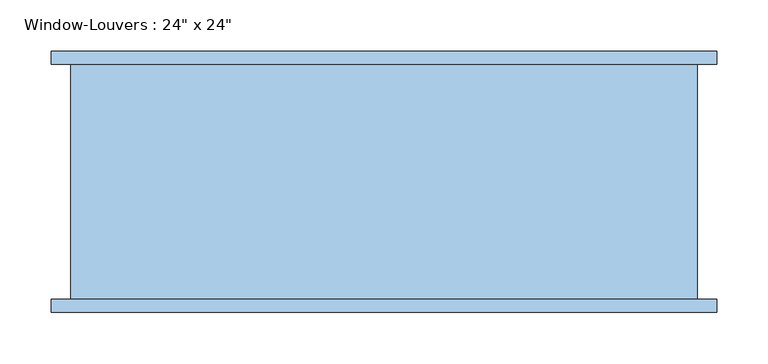
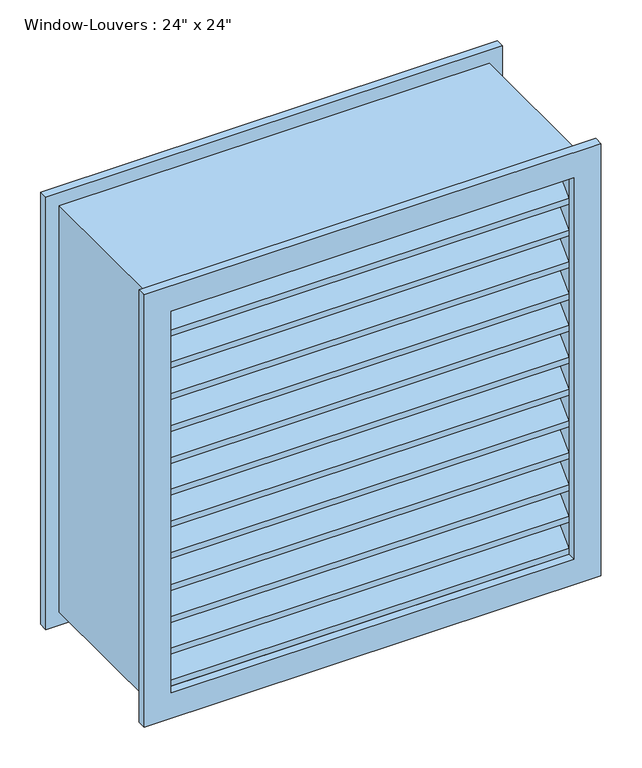
"""IFC4 building model written with IfcOpenShell, lengths in millimetres: window geometry."""

from ifc_helpers import new_model, si_unit, frame, origin, place, context, project, spatial, polyline, outline, extrude, source, transform, mapped, element, save


def window_407d3824(model_context):
    return source(origin(), model_context, "Body", "SweptSolid", [
        extrude(outline(polyline([(-107.95, 1419.1754778), (-69.85, 1457.2754778), (-31.75, 1419.1754778), (-31.75, 1410.1952217), (-69.85, 1448.2952217), (-107.95, 1410.1952217), (-107.95, 1419.1754778)])), frame((-285.75, 0.0, 0.0), z_axis=(1.0, 0.0, 0.0), x_axis=(0.0, 1.0, 0.0)), (0.0, 0.0, 1.0), 571.5),
        extrude(outline(polyline([(-107.95, 1371.5009557), (-69.85, 1409.6009557), (-31.75, 1371.5009557), (-31.75, 1362.5206995), (-69.85, 1400.6206995), (-107.95, 1362.5206995), (-107.95, 1371.5009557)])), frame((-285.75, 0.0, 0.0), z_axis=(1.0, 0.0, 0.0), x_axis=(0.0, 1.0, 0.0)), (0.0, 0.0, 1.0), 571.5),
        extrude(outline(polyline([(-107.95, 1323.8264335), (-69.85, 1361.9264335), (-31.75, 1323.8264335), (-31.75, 1314.8461774), (-69.85, 1352.9461774), (-107.95, 1314.8461774), (-107.95, 1323.8264335)])), frame((-285.75, 0.0, 0.0), z_axis=(1.0, 0.0, 0.0), x_axis=(0.0, 1.0, 0.0)), (0.0, 0.0, 1.0), 571.5),
        extrude(outline(polyline([(-107.95, 1276.1519113), (-69.85, 1314.2519113), (-31.75, 1276.1519113), (-31.75, 1267.1716552), (-69.85, 1305.2716552), (-107.95, 1267.1716552), (-107.95, 1276.1519113)])), frame((-285.75, 0.0, 0.0), z_axis=(1.0, 0.0, 0.0), x_axis=(0.0, 1.0, 0.0)), (0.0, 0.0, 1.0), 571.5),
        extrude(outline(polyline([(-107.95, 1228.4773891), (-69.85, 1266.5773891), (-31.75, 1228.4773891), (-31.75, 1219.497133), (-69.85, 1257.597133), (-107.95, 1219.497133), (-107.95, 1228.4773891)])), frame((-285.75, 0.0, 0.0), z_axis=(1.0, 0.0, 0.0), x_axis=(0.0, 1.0, 0.0)), (0.0, 0.0, 1.0), 571.5),
        extrude(outline(polyline([(-107.95, 1180.802867), (-69.85, 1218.902867), (-31.75, 1180.802867), (-31.75, 1171.8226109), (-69.85, 1209.9226109), (-107.95, 1171.8226109), (-107.95, 1180.802867)])), frame((-285.75, 0.0, 0.0), z_axis=(1.0, 0.0, 0.0), x_axis=(0.0, 1.0, 0.0)), (0.0, 0.0, 1.0), 571.5),
        extrude(outline(polyline([(-107.95, 1133.1283448), (-69.85, 1171.2283448), (-31.75, 1133.1283448), (-31.75, 1124.1480887), (-69.85, 1162.2480887), (-107.95, 1124.1480887), (-107.95, 1133.1283448)])), frame((-285.75, 0.0, 0.0), z_axis=(1.0, 0.0, 0.0), x_axis=(0.0, 1.0, 0.0)), (0.0, 0.0, 1.0), 571.5),
        extrude(outline(polyline([(-107.95, 1085.4538226), (-69.85, 1123.5538226), (-31.75, 1085.4538226), (-31.75, 1076.4735665), (-69.85, 1114.5735665), (-107.95, 1076.4735665), (-107.95, 1085.4538226)])), frame((-285.75, 0.0, 0.0), z_axis=(1.0, 0.0, 0.0), x_axis=(0.0, 1.0, 0.0)), (0.0, 0.0, 1.0), 571.5),
        extrude(outline(polyline([(-107.95, 1037.7793005), (-69.85, 1075.8793005), (-31.75, 1037.7793005), (-31.75, 1028.7990443), (-69.85, 1066.8990443), (-107.95, 1028.7990443), (-107.95, 1037.7793005)])), frame((-285.75, 0.0, 0.0), z_axis=(1.0, 0.0, 0.0), x_axis=(0.0, 1.0, 0.0)), (0.0, 0.0, 1.0), 571.5),
        extrude(outline(polyline([(-107.95, 990.1047783), (-69.85, 1028.2047783), (-31.75, 990.1047783), (-31.75, 981.1245222), (-69.85, 1019.2245222), (-107.95, 981.1245222), (-107.95, 990.1047783)])), frame((-285.75, 0.0, 0.0), z_axis=(1.0, 0.0, 0.0), x_axis=(0.0, 1.0, 0.0)), (0.0, 0.0, 1.0), 571.5),
        extrude(outline(polyline([(-107.95, 1466.85), (-69.85, 1504.95), (-31.75, 1466.85), (-31.75, 1457.8697439), (-69.85, 1495.9697439), (-107.95, 1457.8697439), (-107.95, 1466.85)])), frame((-285.75, 0.0, 0.0), z_axis=(1.0, 0.0, 0.0), x_axis=(0.0, 1.0, 0.0)), (0.0, 0.0, 1.0), 571.5),
        extrude(outline(polyline([(-107.95, 942.4302561), (-69.85, 980.5302561), (-31.75, 942.4302561), (-31.75, 933.45), (-69.85, 971.55), (-107.95, 933.45), (-107.95, 942.4302561)])), frame((-285.75, 0.0, 0.0), z_axis=(1.0, 0.0, 0.0), x_axis=(0.0, 1.0, 0.0)), (0.0, 0.0, 1.0), 571.5),
        extrude(outline(polyline([(1524.0, 304.8), (1524.0, -304.8), (914.4, -304.8), (914.4, 304.8), (1524.0, 304.8)]), holes=[polyline([(1504.95, 285.75), (933.45, 285.75), (933.45, -285.75), (1504.95, -285.75), (1504.95, 285.75)])]), frame((0.0, -107.95, 0.0), z_axis=(0.0, 1.0, 0.0), x_axis=(0.0, 0.0, 1.0)), (0.0, 0.0, 1.0), 228.6),
        extrude(outline(polyline([(1543.05, 323.85), (1543.05, -323.85), (895.35, -323.85), (895.35, 323.85), (1543.05, 323.85)]), holes=[polyline([(1504.95, 285.75), (933.45, 285.75), (933.45, -285.75), (1504.95, -285.75), (1504.95, 285.75)])]), frame((0.0, 120.65, 0.0), z_axis=(0.0, 1.0, 0.0), x_axis=(0.0, 0.0, 1.0)), (0.0, 0.0, 1.0), 12.7),
        extrude(outline(polyline([(1543.05, -323.85), (895.35, -323.85), (895.35, 323.85), (1543.05, 323.85), (1543.05, -323.85)]), holes=[polyline([(1504.95, -285.75), (1504.95, 285.75), (933.45, 285.75), (933.45, -285.75), (1504.95, -285.75)])]), frame((0.0, -120.65, 0.0), z_axis=(0.0, 1.0, 0.0), x_axis=(0.0, 0.0, 1.0)), (0.0, 0.0, 1.0), 12.7),
    ])


if __name__ == "__main__":
    model = new_model("IFC4")
    model_context = context("Model", 3, world=origin())
    ifc_project = project(units=[si_unit("LENGTHUNIT", "METRE", prefix="MILLI")], contexts=[model_context])
    site = spatial("IfcSite", under=ifc_project)
    building = spatial("IfcBuilding", under=site)
    placement = place(None, origin())
    window_shape = window_407d3824(model_context)
    element("IfcWindow", 1, ObjectType="Window-Louvers : 24\" x 24\"", at=placement, inside=building, context=model_context, shape_type="MappedRepresentation", body=[
        mapped(window_shape, transform((0.0, 0.0, 0.0), x_axis=(1.0, 0.0, 0.0), y_axis=(0.0, 1.0, 0.0), z_axis=(0.0, 0.0, 1.0))),
    ])
    save(model, "model.ifc")

# Revit data of these elements
# Type "Window-Louvers : 24\" x 24\""
#   Type Mark = "22"
#   Construction Type Id = "GSP4R"
#   Assembly Code = "B20"
#   Analytic Construction = "1/8 in Pilkington single glazing"
#   Visual Light Transmittance = 0.9
#   Thermal Resistance (R) = 1.53941 (h·ft²·°F)/BTU
#   Solar Heat Gain Coefficient = 0.78
#   Max Height = 1' - 11.74264"
#   Height = 2' - 0"
#   Heat Transfer Coefficient (U) = 0.6496 BTU/(h·ft²·°F)
#   Blade Width [instance default] = 1' - 10 1/2"
#   Blade Vertical Thickness = 0' - 0.35355"
#   Blade Thickness = 0' - 0 1/4"
#   Blade Spacing = 0' - 1 1/2"
#   Blade Height = 0' - 1.85355"
#   Blade Depth = 0' - 3"
#   Blade Angle = 45.00°
#   Default Sill Height = 3' - 0"
#   Trim Projection_Exterior = 0' - 0 1/2"
#   Trim Projection_Interior = 0' - 0 1/2"
#   Trim Width_Exterior = 0' - 1 1/2"
#   Trim Width_Interior = 0' - 1 1/2"
#   Width = 2' - 0"
#   Max Blade Count = 12
#   Define Thermal Properties by = 1
#   Blade Count = 12
#   Frame Material = Birch
#   Louver Material = Birch
#   Trim Exterior Material = Birch
#   Trim Interior Material = Birch
#   Wall Closure = (empty or 0)
# Element 1 (IfcWindow, "Window-Louvers : 24\" x 24\"")
#   Materials on its faces: "Birch"
# Materials
#   "Birch": class "Wood", colour RGB 224 178 126, transparency 0, Description = "Betula Alleghaniensis", Cost = 0
